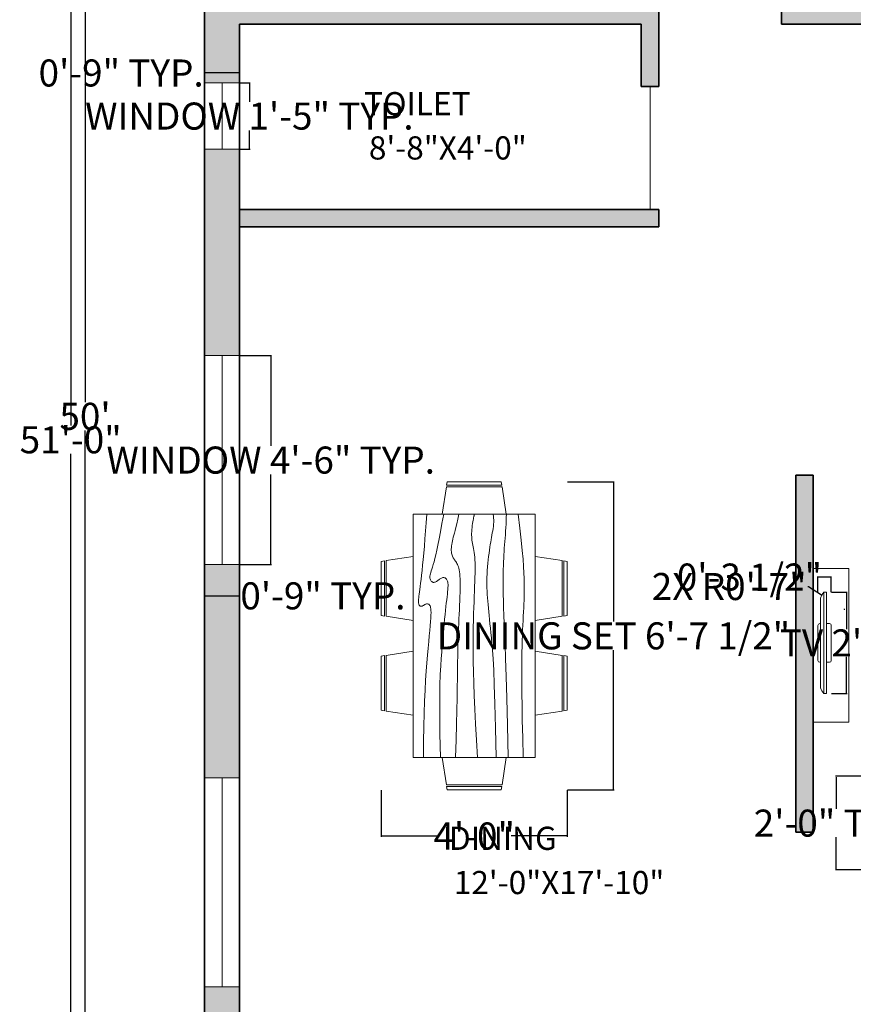
# Model space of a CAD drawing. Units: inches. Extents: x 136 to 672, y -412 to 279.
# Tile 2 of 6: x 136 to 351, y -213 to 42. Entities that reach past the tile are written whole.
import ezdxf

# ---------------------------------------------------------------- set-up
doc = ezdxf.new("R2010")
doc.units = ezdxf.units.IN
doc.header["$MEASUREMENT"] = 0
for name, color, linetype, lineweight in [('A-ANNO-DIMS', 12, 'Continuous', 18), ('A-AREA-IDEN', 7, 'Continuous', 18), ('A-DOOR', 4, 'Continuous', 18), ('A-EQPM', 8, 'Continuous', 18), ('A-FLOR-CASE', 252, 'Continuous', 18), ('A-WALL-PATT', 244, 'Continuous', 9), ('furniture', 252, 'Continuous', 18), ('walls', 253, 'Continuous', 35), ('windows', 171, 'Continuous', 18)]:
    doc.layers.add(name, color=color, linetype=linetype, lineweight=lineweight)
doc.styles.get("Standard").update_dxf_attribs({"font": 'arial.ttf'})
doc.dimstyles.get("Standard").update_dxf_attribs({"dimtxt": 7, "dimasz": 0.18, "dimexe": 0.18, "dimexo": 0.0625, "dimgap": 0.09, "dimtad": 0, "dimtih": 1, "dimtoh": 1, "dimzin": 0, "dimdsep": 46, "dimlunit": 3, "dimtxsty": 'Standard', "dimcen": 0.09, "dimadec": 0, "dimazin": 0, "dimtfac": 1, "dimtofl": 0, "dimtmove": 0, "dimatfit": 3, "dimfxl": 1, "dimtolj": 1, "dimtzin": 0, "dimarcsym": 0})

# ---------------------------------------------------------------- blocks, each defined once
blk = doc.blocks.new('Dining Set - 36 x 72 in.')
for p, q in [((-22, 27.5), (-22.1562, 26.50042)), ((-5.8416, 26.5), (-22.1534, 26.5)), ((-22, 27.5), (-6, 27.5)), ((-5.8437, 26.49966), (-6, 27.5)), ((6, 27.5), (5.8438, 26.50042)), ((22.1584, 26.5), (5.8466, 26.5)), ((6, 27.5), (22, 27.5)), ((22.1563, 26.49966), (22, 27.5)), ((-22.2343, 26.00059), (-23.4847, 17.99762)), ((-22.2304, 26), (-5.7608, 26)), ((-4.5152, 17.99762), (-5.7655, 25.99926)), ((5.7657, 26.00059), (4.5153, 17.99762)), ((5.7696, 26), (22.2392, 26)), ((23.4848, 17.99762), (22.2345, 25.99926)), ((36, 18), (-36, 18)), ((-36, 18), (-36, -18)), ((36, -18), (36, 18)), ((-44.0006, 8.23428), (-35.9976, 9.48474)), ((44.0006, 8.23428), (35.9976, 9.48474)), ((-45.5, 8), (-44.5004, 8.15617)), ((-45.5, 8), (-45.5, -8)), ((-44.5, -8.15843), (-44.5, 8.15338)), ((-44, 8.23041), (-44, -8.23915)), ((44, 8.23041), (44, -8.23915)), ((44.5, -8.15843), (44.5, 8.15338)), ((45.5, 8), (44.5005, 8.15617)), ((45.5, 8), (45.5, -8)), ((-44.4997, -8.15631), (-45.5, -8)), ((-35.9976, -9.48476), (-43.9993, -8.2345)), ((35.9976, -9.48476), (43.9993, -8.2345)), ((44.4997, -8.15631), (45.5, -8)), ((-36, -18), (36, -18)), ((-22.2343, -26.0006), (-23.4847, -17.99762)), ((-4.5152, -17.99762), (-5.7655, -25.99928)), ((5.7657, -26.0006), (4.5153, -17.99762)), ((23.4848, -17.99762), (22.2345, -25.99928)), ((-22.2304, -26), (-5.7608, -26)), ((5.7696, -26), (22.2392, -26)), ((-22, -27.5), (-22.1562, -26.50044)), ((-5.8416, -26.5), (-22.1534, -26.5)), ((-22, -27.5), (-6, -27.5)), ((-5.8437, -26.49967), (-6, -27.5)), ((6, -27.5), (5.8438, -26.50044)), ((22.1584, -26.5), (5.8466, -26.5)), ((6, -27.5), (22, -27.5)), ((22.1563, -26.49967), (22, -27.5))]:
    blk.add_line(p, q)
for points in [[(-36, 15), (-31.1772, 14.97754), (-26.8079, 14.91406), (-22.8538, 14.81543), (-19.276, 14.6875), (-16.0362, 14.53613), (-13.0957, 14.36718), (-10.4159, 14.18652), (-7.9583, 14), (-5.6904, 13.81315), (-3.6035, 13.63021), (-1.6954, 13.45508), (0.0365, 13.29166), (1.5945, 13.14388), (2.9811, 13.01562), (4.1988, 12.9108), (5.25, 12.83333), (6.1393, 12.78613), (6.8802, 12.76823), (7.4883, 12.77767), (7.9792, 12.8125), (8.3685, 12.87077), (8.6719, 12.95052), (8.9049, 13.0498), (9.0833, 13.16666), (9.2205, 13.29899), (9.3216, 13.44401), (9.3895, 13.59879), (9.4271, 13.76041), (9.4373, 13.92594), (9.4232, 14.09245), (9.3875, 14.257), (9.3333, 14.41666), (9.2638, 14.56917), (9.1836, 14.71484), (9.0975, 14.85465), (9.0104, 14.98958), (8.9272, 15.1206), (8.8529, 15.2487), (8.7922, 15.37483), (8.75, 15.5), (8.7305, 15.62467), (8.7344, 15.74739), (8.7617, 15.86621), (8.8125, 15.97916), (8.8867, 16.08431), (8.9844, 16.17968), (9.1055, 16.26334), (9.25, 16.33333), (9.4189, 16.38802), (9.6172, 16.42708), (9.8506, 16.45052), (10.125, 16.45833), (10.4463, 16.45052), (10.8203, 16.42708), (11.2529, 16.38802), (11.75, 16.33333), (12.3184, 16.26318), (12.9694, 16.17838), (13.7151, 16.07991), (14.5677, 15.96875), (15.5395, 15.84586), (16.6426, 15.71224), (17.8893, 15.56884), (19.2917, 15.41666), (20.859, 15.25667), (22.5879, 15.08984), (24.4721, 14.91715), (26.5052, 14.73958), (28.6809, 14.5581), (30.9929, 14.3737), (33.4347, 14.18733), (36, 14)], [(-36, 10), (-28.9766, 10.14274), (-23.1725, 10.20442), (-18.4241, 10.19775), (-14.5677, 10.13541), (-11.4399, 10.03011), (-8.877, 9.89453), (-6.7154, 9.74137), (-4.7917, 9.58333), (-2.9698, 9.43082), (-1.2246, 9.28515), (0.4415, 9.14534), (2.026, 9.01041), (3.5266, 8.87939), (4.9408, 8.7513), (6.266, 8.62516), (7.5, 8.5), (8.6411, 8.37549), (9.6914, 8.2539), (10.6538, 8.13818), (11.5312, 8.03125), (12.3267, 7.93603), (13.043, 7.85547), (13.6831, 7.79248), (14.25, 7.75), (14.7471, 7.7303), (15.1797, 7.73307), (15.5537, 7.75732), (15.875, 7.80208), (16.1494, 7.86637), (16.3828, 7.94922), (16.5811, 8.04964), (16.75, 8.16666), (16.8944, 8.29915), (17.0143, 8.44531), (17.1089, 8.60319), (17.1771, 8.77083), (17.218, 8.94629), (17.2305, 9.1276), (17.2137, 9.31282), (17.1667, 9.5), (17.0895, 9.6875), (16.987, 9.875), (16.8649, 10.0625), (16.7292, 10.25), (16.5856, 10.4375), (16.4401, 10.625), (16.2985, 10.8125), (16.1667, 11), (16.05, 11.18733), (15.9518, 11.3737), (15.8752, 11.5581), (15.8229, 11.73958), (15.798, 11.91715), (15.8034, 12.08984), (15.842, 12.25667), (15.9167, 12.41666), (16.0295, 12.56836), (16.1784, 12.70833), (16.3605, 12.83268), (16.5729, 12.9375), (16.8127, 13.01888), (17.0768, 13.07291), (17.3625, 13.0957), (17.6667, 13.08333), (17.9894, 13.03312), (18.3418, 12.94726), (18.7382, 12.82918), (19.1927, 12.68229), (19.7195, 12.51001), (20.3327, 12.31575), (21.0465, 12.10294), (21.875, 11.875), (22.8357, 11.63354), (23.959, 11.37304), (25.2786, 11.08618), (26.8282, 10.76562), (28.6414, 10.40405), (30.752, 9.99414), (33.1936, 9.52856), (36, 9)], [(-36, 5.5), (-30.7157, 5.3348), (-26.069, 5.20963), (-21.9946, 5.11767), (-18.4271, 5.05208), (-15.3009, 5.00602), (-12.5508, 4.97265), (-10.1112, 4.94515), (-7.9167, 4.91666), (-5.909, 4.88167), (-4.0586, 4.83984), (-2.3429, 4.79215), (-0.7396, 4.73958), (0.7739, 4.6831), (2.22, 4.6237), (3.6213, 4.56233), (5, 4.5), (6.373, 4.43782), (7.7344, 4.3776), (9.0723, 4.32129), (10.375, 4.27083), (11.6309, 4.22819), (12.8281, 4.19531), (13.9551, 4.17415), (15, 4.16666), (15.954, 4.17448), (16.819, 4.19791), (17.6001, 4.23698), (18.3021, 4.29166), (18.9299, 4.36198), (19.4883, 4.44791), (19.9823, 4.54948), (20.4167, 4.66666), (20.7969, 4.79899), (21.1302, 4.94401), (21.4245, 5.09879), (21.6875, 5.26041), (21.9271, 5.42594), (22.1511, 5.59245), (22.3672, 5.757), (22.5834, 5.91666), (22.8065, 6.06868), (23.0404, 6.21093), (23.2879, 6.34147), (23.5521, 6.45833), (23.8358, 6.55957), (24.142, 6.64323), (24.4735, 6.70735), (24.8334, 6.75), (25.2235, 6.76969), (25.642, 6.76692), (26.0858, 6.74267), (26.5521, 6.69791), (27.0379, 6.63362), (27.5404, 6.55078), (28.0565, 6.45036), (28.5834, 6.33333), (29.1242, 6.19987), (29.7071, 6.04687), (30.3661, 5.87044), (31.1354, 5.66666), (32.0493, 5.43164), (33.142, 5.16146), (34.4475, 4.85221), (36, 4.5)], [(-36, -1), (-30.7915, -0.6591), (-26.0195, -0.38216), (-21.6519, -0.16284), (-17.6563, 0.00521), (-14.0005, 0.12833), (-10.6523, 0.21289), (-7.5796, 0.26522), (-4.75, 0.29166), (-2.134, 0.29793), (0.2878, 0.28711), (2.5317, 0.26163), (4.6146, 0.22396), (6.5529, 0.17651), (8.3633, 0.12174), (10.0623, 0.06209), (11.6667, 0), (13.1899, -0.06201), (14.6341, -0.1211), (15.9982, -0.17432), (17.2813, -0.21875), (18.4823, -0.25147), (19.6003, -0.26953), (20.6343, -0.27002), (21.5834, -0.25), (22.4481, -0.20768), (23.2357, -0.14584), (23.9549, -0.06836), (24.6146, 0.02083), (25.2235, 0.11784), (25.7904, 0.21875), (26.3241, 0.31966), (26.8334, 0.41666), (27.3265, 0.50618), (27.8099, 0.58593), (28.2894, 0.65397), (28.7709, 0.70833), (29.2601, 0.74707), (29.763, 0.76823), (30.2855, 0.76985), (30.8334, 0.75), (31.4088, 0.70784), (31.9994, 0.64713), (32.589, 0.57275), (33.1615, 0.48958), (33.7008, 0.4025), (34.1908, 0.3164), (34.6153, 0.23616), (34.9584, 0.16666), (35.2099, 0.11165), (35.3848, 0.07031), (35.504, 0.04069), (35.5886, 0.02083), (35.6594, 0.00879), (35.7377, 0.0026), (35.8442, 0.00032), (36, 0)], [(-36, -6.5), (-27.1843, -6.31267), (-20.084, -6.1263), (-14.469, -5.9419), (-10.1094, -5.76042), (-6.7752, -5.58285), (-4.2363, -5.41016), (-2.2629, -5.24333), (-0.625, -5.08334), (0.8708, -4.93099), (2.2715, -4.78646), (3.5872, -4.64974), (4.8281, -4.52084), (6.0046, -4.39974), (7.127, -4.28646), (8.2053, -4.18099), (9.25, -4.08334), (10.2705, -3.99382), (11.2734, -3.91407), (12.2647, -3.84603), (13.25, -3.79167), (14.2354, -3.75293), (15.2266, -3.73177), (16.2295, -3.73015), (17.25, -3.75), (18.2912, -3.79248), (19.3451, -3.85547), (20.4009, -3.93604), (21.4479, -4.03125), (22.4754, -4.13819), (23.4727, -4.25391), (24.4289, -4.37549), (25.3334, -4.5), (26.1785, -4.62492), (26.9694, -4.74935), (27.7145, -4.87281), (28.4219, -4.99479), (29.1, -5.11483), (29.7572, -5.23242), (30.4016, -5.34709), (31.0417, -5.45834), (31.6837, -5.56437), (32.3262, -5.65821), (32.9658, -5.73153), (33.599, -5.77604), (34.2224, -5.78345), (34.8327, -5.74545), (35.4264, -5.65373), (36, -5.5)], [(-36, -10), (-26.4022, -9.81299), (-18.4675, -9.62891), (-11.9839, -9.45069), (-6.7396, -9.28125), (-2.5226, -9.12354), (0.8789, -8.98047), (3.6769, -8.85498), (6.0833, -8.75), (8.2767, -8.66765), (10.3021, -8.60677), (12.1712, -8.56543), (13.8958, -8.54167), (15.4876, -8.53353), (16.9583, -8.53907), (18.3197, -8.55632), (19.5834, -8.58334), (20.7616, -8.61841), (21.8685, -8.66081), (22.9188, -8.71004), (23.9271, -8.76563), (24.9081, -8.82707), (25.8763, -8.89388), (26.8465, -8.96558), (27.8334, -9.04167), (28.8474, -9.12118), (29.8828, -9.20117), (30.93, -9.27824), (31.9792, -9.34896), (33.0205, -9.40991), (34.0443, -9.45768), (35.0407, -9.48885), (36, -9.5)], [(-36, -14.5), (-30.0881, -14.33513), (-25.0332, -14.21224), (-20.7312, -14.12647), (-17.0781, -14.07292), (-13.97, -14.04671), (-11.3027, -14.04297), (-8.9724, -14.05681), (-6.875, -14.08334), (-4.9224, -14.11833), (-3.0905, -14.16016), (-1.3709, -14.20785), (0.2448, -14.26042), (1.7647, -14.3169), (3.1973, -14.3763), (4.5507, -14.43767), (5.8333, -14.5), (7.0554, -14.5621), (8.235, -14.62175), (9.3922, -14.67652), (10.5469, -14.72396), (11.7192, -14.76164), (12.929, -14.78711), (14.1965, -14.79794), (15.5417, -14.79167), (16.9933, -14.76424), (18.6152, -14.70508), (20.4804, -14.60197), (22.6615, -14.44271), (25.2312, -14.21509), (28.2624, -13.9069), (31.8277, -13.50594), (36, -13)]]:
    blk.add_lwpolyline(points)
blk = doc.blocks.new('dining area')
at = {"layer": 'furniture', "xscale": 0.6659924291999282, "yscale": 0.6659924291999282, "zscale": 0.6659924291999282, "rotation": 90}
blk.add_blockref('Dining Set - 36 x 72 in.', (-0.44, 20.51), dxfattribs=at)
blk = doc.blocks.new('PLASMA-LARGE')
at = {"layer": 'furniture'}
for p, q in [((-7.26, 0), (7.26, 0)), ((-21, -2.5), (21, -2.5)), ((-21, -2.5), (-21, -3.5)), ((-21, -3.5), (21, -3.5)), ((-18.61, -1), (18.61, -1)), ((-8, -1), (-8, -0.74)), ((-8, -3.5), (-8, -4.76)), ((8, -1), (8, -0.74)), ((8, -3.5), (8, -4.76)), ((21, -2.5), (21, -3.5)), ((-7.26, -5.5), (7.26, -5.5))]:
    blk.add_line(p, q, dxfattribs=at)
for centre, radius, start, end in [((-7.26, -0.74), 0.744, 90, 180), ((7.26, -0.74), 0.744, 0, 90), ((-13.97, -11.05), 11.07, 114.7602, 129.4175), ((13.97, -11.05), 11.07, 50.5825, 65.2398), ((-7.26, -4.76), 0.744, 180, 270), ((7.26, -4.76), 0.744, 270, 0)]:
    blk.add_arc(centre, radius, start, end, dxfattribs=at)
blk = doc.blocks.new('*D19')
at = {"layer": 'A-ANNO-DIMS', "color": 0, "lineweight": -2, "transparency": 16777216}
for p, q in [((152.44, 239.56), (152.7, 239.56)), ((152.52, 239.38), (152.52, -56.77)), ((152.52, -360.26), (152.52, -64.1)), ((152.44, -360.44), (152.7, -360.44))]:
    blk.add_line(p, q, dxfattribs=at)
at = {"layer": 'A-ANNO-DIMS', "color": 0, "transparency": 16777216}
for points in [[(152.49, 239.38), (152.55, 239.38), (152.52, 239.56)], [(152.49, -360.26), (152.55, -360.26), (152.52, -360.44)]]:
    blk.add_solid(points, dxfattribs=at)
at = {"layer": 'Defpoints', "color": 0, "transparency": 16777216}
for p in [(152.38, 239.56), (152.38, -360.44), (152.52, -360.44)]:
    blk.add_point(p, dxfattribs=at)
at = {"layer": 'A-ANNO-DIMS', "color": 0, "transparency": 16777216, "insert": (152.52, -60.44), "char_height": 7, "attachment_point": 5}
blk.add_mtext("\\A1;50'", dxfattribs=at)
blk = doc.blocks.new('WIN-54')
for p, q in [((0, 54.05), (9, 54.05)), ((0, 0), (0, 54.05)), ((0, 54.05), (4.5, 54.05)), ((4.5, 54.05), (4.5, 0)), ((9, 54.05), (9, 0)), ((9, 0), (0, 0))]:
    blk.add_line(p, q)
blk = doc.blocks.new('WIN-17')
for p, q in [((0, 9), (0, 0)), ((17.15, 9), (0, 9)), ((0, 9), (0, 4.5)), ((17.15, 0), (17.15, 9)), ((0, 4.5), (17.15, 4.5)), ((0, 0), (17.15, 0))]:
    blk.add_line(p, q)
blk = doc.blocks.new('*D35')
at = {"layer": 'A-ANNO-DIMS', "color": 0, "lineweight": -2, "transparency": 16777216}
for p, q in [((345.66, -105.96), (349.71, -105.96)), ((349.53, -106.14), (349.53, -115.47)), ((349.53, -132), (349.53, -122.68)), ((345.66, -132.18), (349.71, -132.18))]:
    blk.add_line(p, q, dxfattribs=at)
at = {"layer": 'A-ANNO-DIMS', "color": 0, "transparency": 16777216}
for points in [[(349.5, -106.14), (349.56, -106.14), (349.53, -105.96)], [(349.5, -132), (349.56, -132), (349.53, -132.18)]]:
    blk.add_solid(points, dxfattribs=at)
at = {"layer": 'Defpoints', "color": 0, "transparency": 16777216}
for p in [(345.6, -105.96), (349.53, -105.96), (345.6, -132.18)]:
    blk.add_point(p, dxfattribs=at)
at = {"layer": 'A-ANNO-DIMS', "color": 0, "transparency": 16777216, "insert": (349.53, -119.07), "char_height": 7, "attachment_point": 5}
blk.add_mtext('\\A1;TV 2\'-2"', dxfattribs=at)
blk = doc.blocks.new('*D36')
at = {"layer": 'A-ANNO-DIMS', "color": 0, "lineweight": -2, "transparency": 16777216}
for p, q in [((342.17, -105.9), (342.17, -101.85)), ((345.6, -105.9), (345.6, -101.85)), ((342.17, -102.03), (341.99, -102.03)), ((345.42, -102.03), (342.35, -102.03))]:
    blk.add_line(p, q, dxfattribs=at)
at = {"layer": 'A-ANNO-DIMS', "color": 0, "transparency": 16777216}
for points in [[(342.35, -102), (342.35, -102.06), (342.17, -102.03)], [(345.42, -102), (345.42, -102.06), (345.6, -102.03)]]:
    blk.add_solid(points, dxfattribs=at)
at = {"layer": 'Defpoints', "color": 0, "transparency": 16777216}
for p in [(342.17, -102.03), (342.17, -105.96), (345.6, -105.96)]:
    blk.add_point(p, dxfattribs=at)
at = {"layer": 'A-ANNO-DIMS', "color": 0, "transparency": 16777216, "insert": (324.44, -102.03), "char_height": 7, "attachment_point": 5}
blk.add_mtext('\\A1;0\'-3 1/2"', dxfattribs=at)
blk = doc.blocks.new('*D38')
at = {"layer": 'A-ANNO-DIMS', "color": 0, "lineweight": -2, "transparency": 16777216}
for p, q in [((358.4, -153.59), (346.74, -153.59)), ((346.92, -153.77), (346.92, -162.04)), ((346.92, -177.64), (346.92, -169.37)), ((358.4, -177.82), (346.74, -177.82))]:
    blk.add_line(p, q, dxfattribs=at)
at = {"layer": 'A-ANNO-DIMS', "color": 0, "transparency": 16777216}
for points in [[(346.89, -153.77), (346.95, -153.77), (346.92, -153.59)], [(346.89, -177.64), (346.95, -177.64), (346.92, -177.82)]]:
    blk.add_solid(points, dxfattribs=at)
at = {"layer": 'Defpoints', "color": 0, "transparency": 16777216}
for p in [(346.92, -153.59), (358.47, -153.59), (358.47, -177.82)]:
    blk.add_point(p, dxfattribs=at)
at = {"layer": 'A-ANNO-DIMS', "color": 0, "transparency": 16777216, "insert": (346.92, -165.7), "char_height": 7, "attachment_point": 5}
blk.add_mtext('\\A1;2\'-0" TYP.', dxfattribs=at)
blk = doc.blocks.new('*D45')
at = {"layer": 'A-ANNO-DIMS', "color": 0, "lineweight": -2, "transparency": 16777216}
for p, q in [((277.37, -77.4), (289.44, -77.4)), ((289.26, -77.58), (289.26, -113.53)), ((289.26, -156.9), (289.26, -120.95)), ((277.37, -157.08), (289.44, -157.08))]:
    blk.add_line(p, q, dxfattribs=at)
at = {"layer": 'A-ANNO-DIMS', "color": 0, "transparency": 16777216}
for points in [[(289.23, -77.58), (289.29, -77.58), (289.26, -77.4)], [(289.23, -156.9), (289.29, -156.9), (289.26, -157.08)]]:
    blk.add_solid(points, dxfattribs=at)
at = {"layer": 'Defpoints', "color": 0, "transparency": 16777216}
for p in [(277.3, -77.4), (289.26, -77.4), (277.3, -157.08)]:
    blk.add_point(p, dxfattribs=at)
at = {"layer": 'A-ANNO-DIMS', "color": 0, "transparency": 16777216, "insert": (289.26, -117.24), "char_height": 7, "attachment_point": 5}
blk.add_mtext('\\A1;DINING SET 6\'-7 1/2"', dxfattribs=at)
blk = doc.blocks.new('*D46')
at = {"layer": 'A-ANNO-DIMS', "color": 0, "lineweight": -2, "transparency": 16777216}
for p, q in [((229.15, -157.14), (229.15, -169.21)), ((277.3, -157.14), (277.3, -169.21)), ((229.33, -169.03), (243.69, -169.03)), ((277.12, -169.03), (262.76, -169.03))]:
    blk.add_line(p, q, dxfattribs=at)
at = {"layer": 'A-ANNO-DIMS', "color": 0, "transparency": 16777216}
for points in [[(229.33, -169), (229.33, -169.06), (229.15, -169.03)], [(277.12, -169), (277.12, -169.06), (277.3, -169.03)]]:
    blk.add_solid(points, dxfattribs=at)
at = {"layer": 'Defpoints', "color": 0, "transparency": 16777216}
for p in [(229.15, -157.08), (277.3, -157.08), (277.3, -169.03)]:
    blk.add_point(p, dxfattribs=at)
at = {"layer": 'A-ANNO-DIMS', "color": 0, "transparency": 16777216, "insert": (253.23, -169.03), "char_height": 7, "attachment_point": 5}
blk.add_mtext('\\A1;4\'-0"', dxfattribs=at)
blk = doc.blocks.new('*D47')
at = {"layer": 'A-ANNO-DIMS', "color": 0, "lineweight": -2, "transparency": 16777216}
for p, q in [((192.53, -44.73), (200.75, -44.73)), ((200.57, -44.91), (200.57, -68.05)), ((200.57, -98.6), (200.57, -75.47)), ((192.53, -98.78), (200.75, -98.78))]:
    blk.add_line(p, q, dxfattribs=at)
at = {"layer": 'A-ANNO-DIMS', "color": 0, "transparency": 16777216}
for points in [[(200.54, -44.91), (200.6, -44.91), (200.57, -44.73)], [(200.54, -98.6), (200.6, -98.6), (200.57, -98.78)]]:
    blk.add_solid(points, dxfattribs=at)
at = {"layer": 'Defpoints', "color": 0, "transparency": 16777216}
for p in [(192.46, -44.73), (200.57, -44.73), (192.46, -98.78)]:
    blk.add_point(p, dxfattribs=at)
at = {"layer": 'A-ANNO-DIMS', "color": 0, "transparency": 16777216, "insert": (200.57, -71.76), "char_height": 7, "attachment_point": 5}
blk.add_mtext('\\A1;WINDOW 4\'-6" TYP.', dxfattribs=at)
blk = doc.blocks.new('*D48')
at = {"layer": 'A-ANNO-DIMS', "color": 0, "lineweight": -2, "transparency": 16777216}
for p, q in [((183.46, -98.84), (183.46, -107.07)), ((192.46, -98.84), (192.46, -107.07)), ((183.64, -106.89), (192.28, -106.89)), ((192.46, -106.89), (192.64, -106.89))]:
    blk.add_line(p, q, dxfattribs=at)
at = {"layer": 'A-ANNO-DIMS', "color": 0, "transparency": 16777216}
for points in [[(183.64, -106.86), (183.64, -106.92), (183.46, -106.89)], [(192.28, -106.86), (192.28, -106.92), (192.46, -106.89)]]:
    blk.add_solid(points, dxfattribs=at)
at = {"layer": 'Defpoints', "color": 0, "transparency": 16777216}
for p in [(183.46, -98.78), (192.46, -98.78), (192.46, -106.89)]:
    blk.add_point(p, dxfattribs=at)
at = {"layer": 'A-ANNO-DIMS', "color": 0, "transparency": 16777216, "insert": (214.07, -106.89), "char_height": 7, "attachment_point": 5}
blk.add_mtext('\\A1;0\'-9" TYP.', dxfattribs=at)
blk = doc.blocks.new('*D49')
at = {"layer": 'A-ANNO-DIMS', "color": 0, "lineweight": -2, "transparency": 16777216}
for p, q in [((192.53, 25.82), (195.22, 25.82)), ((195.04, 25.64), (195.04, 20.96)), ((195.04, 8.85), (195.04, 13.54)), ((192.53, 8.67), (195.22, 8.67))]:
    blk.add_line(p, q, dxfattribs=at)
at = {"layer": 'A-ANNO-DIMS', "color": 0, "transparency": 16777216}
for points in [[(195.01, 25.64), (195.07, 25.64), (195.04, 25.82)], [(195.01, 8.85), (195.07, 8.85), (195.04, 8.67)]]:
    blk.add_solid(points, dxfattribs=at)
at = {"layer": 'Defpoints', "color": 0, "transparency": 16777216}
for p in [(192.46, 25.82), (195.04, 25.82), (192.46, 8.67)]:
    blk.add_point(p, dxfattribs=at)
at = {"layer": 'A-ANNO-DIMS', "color": 0, "transparency": 16777216, "insert": (195.04, 17.25), "char_height": 7, "attachment_point": 5}
blk.add_mtext('\\A1;WINDOW 1\'-5" TYP.', dxfattribs=at)
blk = doc.blocks.new('*D50')
at = {"layer": 'A-ANNO-DIMS', "color": 0, "lineweight": -2, "transparency": 16777216}
for p, q in [((183.46, 28.4), (183.28, 28.4)), ((183.46, 25.89), (183.46, 28.58)), ((192.28, 28.4), (183.64, 28.4)), ((192.46, 25.89), (192.46, 28.58))]:
    blk.add_line(p, q, dxfattribs=at)
at = {"layer": 'A-ANNO-DIMS', "color": 0, "transparency": 16777216}
for points in [[(183.64, 28.43), (183.64, 28.37), (183.46, 28.4)], [(192.28, 28.43), (192.28, 28.37), (192.46, 28.4)]]:
    blk.add_solid(points, dxfattribs=at)
at = {"layer": 'Defpoints', "color": 0, "transparency": 16777216}
for p in [(183.46, 28.4), (183.46, 25.82), (192.46, 25.82)]:
    blk.add_point(p, dxfattribs=at)
at = {"layer": 'A-ANNO-DIMS', "color": 0, "transparency": 16777216, "insert": (161.86, 28.4), "char_height": 7, "attachment_point": 5}
blk.add_mtext('\\A1;0\'-9" TYP.', dxfattribs=at)
blk = doc.blocks.new('*D56')
at = {"layer": 'A-ANNO-DIMS', "color": 0, "lineweight": -2, "transparency": 16777216}
for p, q in [((183.4, 239.56), (148.63, 239.56)), ((148.81, 239.38), (148.81, -62.84)), ((148.81, -372.4), (148.81, -70.17)), ((219.39, -372.58), (148.63, -372.58))]:
    blk.add_line(p, q, dxfattribs=at)
at = {"layer": 'A-ANNO-DIMS', "color": 0, "transparency": 16777216}
for points in [[(148.78, 239.38), (148.84, 239.38), (148.81, 239.56)], [(148.78, -372.4), (148.84, -372.4), (148.81, -372.58)]]:
    blk.add_solid(points, dxfattribs=at)
at = {"layer": 'Defpoints', "color": 0, "transparency": 16777216}
for p in [(183.46, 239.56), (148.81, -372.58), (219.45, -372.58)]:
    blk.add_point(p, dxfattribs=at)
at = {"layer": 'A-ANNO-DIMS', "color": 0, "transparency": 16777216, "insert": (148.81, -66.51), "char_height": 7, "attachment_point": 5}
blk.add_mtext('\\A1;51\'-0"', dxfattribs=at)
blk = doc.blocks.new('*D58')
at = {"layer": 'A-ANNO-DIMS', "color": 0, "lineweight": -2, "transparency": 16777216}
for p, q in [((339.52, -104.48), (339.7, -104.48)), ((339.7, -104.48), (343.06, -106.59)), ((348.97, -110.35), (349.15, -110.35)), ((349.06, -110.44), (349.06, -110.26))]:
    blk.add_line(p, q, dxfattribs=at)
at = {"layer": 'A-ANNO-DIMS', "color": 0, "transparency": 16777216}
blk.add_solid([(343.07, -106.56), (343.04, -106.61), (343.21, -106.68)], dxfattribs=at)
at = {"layer": 'Defpoints', "color": 0, "transparency": 16777216}
for p in [(343.21, -106.68), (349.06, -110.35)]:
    blk.add_point(p, dxfattribs=at)
at = {"layer": 'A-ANNO-DIMS', "color": 0, "transparency": 16777216, "insert": (319.2, -104.48), "char_height": 7, "attachment_point": 5}
blk.add_mtext('\\A1;2X R0\'-7"', dxfattribs=at)

msp = doc.modelspace()

# ---------------------------------------------------------------- hatches: boundary and pattern name
at = {"layer": 'A-WALL-PATT'}
h = msp.add_hatch(color=256, dxfattribs=at)
h.dxf.hatch_style = 1
h.paths.add_polyline_path([(255.026, 239.565), (183.463, 239.565), (183.463, 125.252), (187.963, 125.252), (192.463, 125.252), (192.463, 230.565), (255.024, 230.565), (255.025, 235.065)])
h.paths.add_polyline_path([(369.355, 239.565), (332.259, 239.565), (332.259, 230.565), (342.463, 230.565), (342.463, 104.521), (346.963, 104.521), (346.963, 230.565), (369.355, 230.565), (369.355, 235.065)])
h.paths.add_polyline_path([(603.463, 239.565), (385.627, 239.565), (385.627, 230.565), (406.963, 230.565), (406.963, 134.565), (371.802, 134.565), (371.802, 130.065), (406.963, 130.065), (406.963, 45.565), (346.963, 45.565), (346.963, 69.395), (342.463, 69.395), (342.463, 45.565), (332.733, 45.565), (332.733, 41.065), (416.87, 41.065), (416.87, 45.565), (411.463, 45.565), (411.463, 230.565), (594.463, 230.565), (594.463, 199.893), (598.963, 199.893), (603.463, 199.893)])
h.paths.add_polyline_path([(603.463, 145.845), (594.463, 145.845), (594.463, 98.065), (524.374, 98.065), (512.275, 97.948), (512.275, 98.065), (484.021, 98.065), (484.021, 93.565), (505.963, 93.565), (594.463, 93.565), (594.463, 80.073), (598.963, 80.073), (603.463, 80.073)], flags=17)
h.paths.add_polyline_path([(457.963, 98.065), (453.463, 98.065), (453.463, 41.065), (594.463, 41.065), (594.463, -67.933), (603.463, -67.933), (603.463, 63.801), (594.463, 63.801), (594.463, 45.565), (510.463, 45.565), (510.463, 65.243), (505.963, 65.243), (505.963, 45.565), (457.963, 45.565)])
h.paths.add_polyline_path([(192.463, 71.205), (183.463, 71.205), (183.463, 25.824), (192.463, 25.824), (192.463, 41.065), (296.463, 41.065), (296.463, 24.884), (300.963, 24.884), (300.963, 45.565), (192.463, 45.565)])
h.paths.add_polyline_path([(300.963, -6.935), (296.463, -6.935), (192.463, -6.935), (192.463, -11.435), (300.963, -11.435)])
h.paths.add_polyline_path([(192.463, 8.674), (183.463, 8.674), (183.463, -44.733), (187.963, -44.733), (192.463, -44.733)])
h.paths.add_polyline_path([(235.886, -349.935), (192.463, -349.935), (192.463, -358.935), (235.886, -358.935)])
h.paths.add_polyline_path([(345.463, -316.935), (361.986, -316.935), (361.986, -307.935), (340.963, -307.935), (340.963, -229.935), (356.354, -229.935), (356.354, -225.435), (336.463, -225.435), (336.463, -349.935), (300.655, -349.935), (300.655, -358.935), (345.463, -358.935)])
h.paths.add_polyline_path([(407.452, -307.935), (403.463, -307.935), (403.463, -225.435), (382.286, -225.435), (382.286, -229.935), (398.963, -229.935), (398.963, -307.935), (379.137, -307.935), (379.137, -316.935), (407.452, -316.935)])
h.paths.add_polyline_path([(470.463, -284.28), (461.463, -284.28), (461.463, -307.935), (461.463, -316.935), (470.463, -316.935)])
h.paths.add_polyline_path([(470.463, -234.435), (480.349, -234.435), (480.349, -225.435), (461.463, -225.435), (461.463, -245.135), (470.463, -245.135)])
h.paths.add_polyline_path([(603.463, -121.943), (594.463, -121.943), (594.463, -225.435), (574.368, -225.435), (574.368, -234.435), (603.463, -234.435)])
h.paths.add_polyline_path([(340.963, -75.678), (336.463, -75.678), (336.463, -168.061), (340.963, -168.061)])
h.paths.add_polyline_path([(468.637, 59.14), (510.671, 59.14), (510.671, 68.331), (468.637, 68.331)], flags=25)
h.paths.add_polyline_path([(192.463, -208.04), (183.463, -208.04), (183.463, -360.435), (192.463, -360.435)])
h.paths.add_polyline_path([(183.463, -153.992), (192.463, -153.992), (192.463, -98.781), (183.463, -98.781)])

# ---------------------------------------------------------------- linework, layer by layer
at = {"layer": 'A-DOOR'}
msp.add_line((298.713, 24.884), (298.713, -6.935), dxfattribs=at)
at = {"layer": 'A-FLOR-CASE'}
for p, q in [((340.963, -99.826), (350.158, -99.826)), ((350.158, -99.826), (350.158, -139.604)), ((350.158, -139.604), (340.963, -139.604))]:
    msp.add_line(p, q, dxfattribs=at)
at = {"layer": 'walls'}
for p, q in [((183.463, -360.435), (183.463, 239.565)), ((300.963, 24.884), (300.963, 45.565)), ((332.733, 45.565), (332.733, 41.065)), ((192.463, -360.435), (192.463, 41.065)), ((192.463, 41.065), (296.463, 41.065)), ((296.463, 24.884), (296.463, 41.065)), ((332.733, 41.065), (416.87, 41.065)), ((296.463, 24.884), (300.963, 24.884)), ((192.463, -6.935), (296.463, -6.935)), ((296.463, -6.935), (300.963, -6.935)), ((300.963, -11.435), (300.963, -6.935)), ((192.463, -11.435), (300.963, -11.435)), ((336.463, -75.678), (340.963, -75.678)), ((336.463, -168.061), (336.463, -75.678)), ((340.963, -168.061), (340.963, -75.678)), ((336.463, -168.061), (340.963, -168.061))]:
    msp.add_line(p, q, dxfattribs=at)
at = {"layer": 'windows'}
for p, q in [((183.463, -208.04), (183.463, -153.992)), ((183.463, -153.992), (192.463, -153.992)), ((187.963, -153.992), (187.963, -208.04)), ((192.463, -153.992), (192.463, -208.04)), ((183.463, -208.04), (192.463, -208.04))]:
    msp.add_line(p, q, dxfattribs=at)

# ---------------------------------------------------------------- block references
at = {"layer": 'A-EQPM', "xscale": 0.6242177563149967, "yscale": 0.6242177563149967, "zscale": 0.6242177563149967, "rotation": 89.99999999999999}
msp.add_blockref('PLASMA-LARGE', (342.166, -119.073), dxfattribs=at)
at = {"layer": 'furniture', "xscale": 1.314690249935364, "yscale": 1.314690249935364, "zscale": 1.314690249935364}
msp.add_blockref('dining area', (253.802, -144.203), dxfattribs=at)
at = {"layer": 'windows', "rotation": 90.00000000000006}
msp.add_blockref('WIN-17', (192.463, 8.674), dxfattribs=at)
at = {"layer": 'windows'}
msp.add_blockref('WIN-54', (183.463, -98.781), dxfattribs=at)

# ---------------------------------------------------------------- texts
at = {"layer": 'A-AREA-IDEN'}
for s, p in [('TOILET', (224.732, 17.458)), ('8\'-8"X4\'-0"', (225.97, 6.011)), ('DINING', (246.692, -172.626)), ('12\'-0"X17\'-10"', (247.93, -184.073))]:
    msp.add_text(s, height=6, dxfattribs=at).set_placement(p)

# ---------------------------------------------------------------- dimensions: what is measured, and where the dimension line sits
at = {"layer": 'A-ANNO-DIMS'}
for base, p1, p2, angle, override, picture, middle in [((148.813, -372.578), (183.463, 239.565), (219.455, -372.578), 90, {"dimdec": 1, "dimlfac": 1, "dimrnd": 0, "dimzin": 1, "dimdsep": 46, "dimlunit": 4, "dimfrac": 2}, '*D56', (148.813, -66.506)), ((152.519, -360.435), (152.38, 239.565), (152.38, -360.435), 90, {"dimclrd": 0, "dimclre": 0, "dimclrt": 0}, '*D19', (152.519, -60.435)), ((342.166, -102.032), (345.6, -105.965), (342.166, -105.965), 180, {"dimdec": 1, "dimlfac": 1, "dimrnd": 0, "dimzin": 1, "dimdsep": 46, "dimlunit": 4, "dimfrac": 2}, '*D36', (324.437, -102.032))]:
    dim = msp.add_linear_dim(base=base, p1=p1, p2=p2, angle=angle, dimstyle='Standard', override=override, dxfattribs=at)
    dim.commit()
    dim.dimension.update_dxf_attribs({"geometry": picture, "text_midpoint": middle})
for base, p1, p2, angle, text, picture, middle in [((183.463, 28.397), (192.463, 25.824), (183.463, 25.824), 180, '<> TYP.', '*D50', (161.858, 28.397)), ((195.0353, 25.8242), (192.4627, 8.6737), (192.4627, 25.8242), 90, 'WINDOW <> TYP.', '*D49', (195.0353, 17.2489)), ((200.57, -44.733), (192.463, -98.781), (192.463, -44.733), 90, 'WINDOW <> TYP.', '*D47', (200.57, -71.757)), ((289.255, -77.404), (277.304, -157.081), (277.304, -77.404), 90, 'DINING SET <>', '*D45', (289.255, -117.242)), ((349.532, -105.965), (345.6, -132.182), (345.6, -105.965), 90, 'TV <>', '*D35', (349.532, -119.073)), ((346.92, -153.588), (358.466, -177.82), (358.466, -153.588), 90, '<> TYP.', '*D38', (346.92, -165.704))]:
    dim = msp.add_linear_dim(base=base, p1=p1, p2=p2, angle=angle, text=text, dimstyle='Standard', override={"dimdec": 1, "dimlfac": 1, "dimrnd": 0, "dimzin": 1, "dimdsep": 46, "dimlunit": 4, "dimfrac": 2}, dxfattribs=at)
    dim.commit()
    dim.dimension.update_dxf_attribs({"geometry": picture, "text_midpoint": middle})
dim = msp.add_radius_dim(center=(349.064, -110.352), mpoint=(343.211, -106.681), text='2X <>', dimstyle='Standard', override={"dimdec": 1, "dimlfac": 1, "dimrnd": 0, "dimzin": 1, "dimdsep": 46, "dimlunit": 4, "dimfrac": 2}, dxfattribs=at)
dim.commit()
dim.dimension.update_dxf_attribs({"geometry": '*D58', "text_midpoint": (319.196, -104.479), "dimtype": 164})
dim = msp.add_linear_dim(base=(192.463, -106.888), p1=(183.463, -98.781), p2=(192.463, -98.781), text='<> TYP.', dimstyle='Standard', override={"dimdec": 1, "dimlfac": 1, "dimrnd": 0, "dimzin": 1, "dimdsep": 46, "dimlunit": 4, "dimfrac": 2}, dxfattribs=at)
dim.commit()
dim.dimension.update_dxf_attribs({"geometry": '*D48', "text_midpoint": (214.067, -106.888)})
dim = msp.add_linear_dim(base=(277.304, -169.033), p1=(229.147, -157.081), p2=(277.304, -157.081), dimstyle='Standard', override={"dimdec": 1, "dimlfac": 1, "dimrnd": 0, "dimzin": 1, "dimdsep": 46, "dimlunit": 4, "dimfrac": 2}, dxfattribs=at)
dim.commit()
dim.dimension.update_dxf_attribs({"geometry": '*D46', "text_midpoint": (253.225, -169.033)})

doc.saveas('drawing.dxf')
